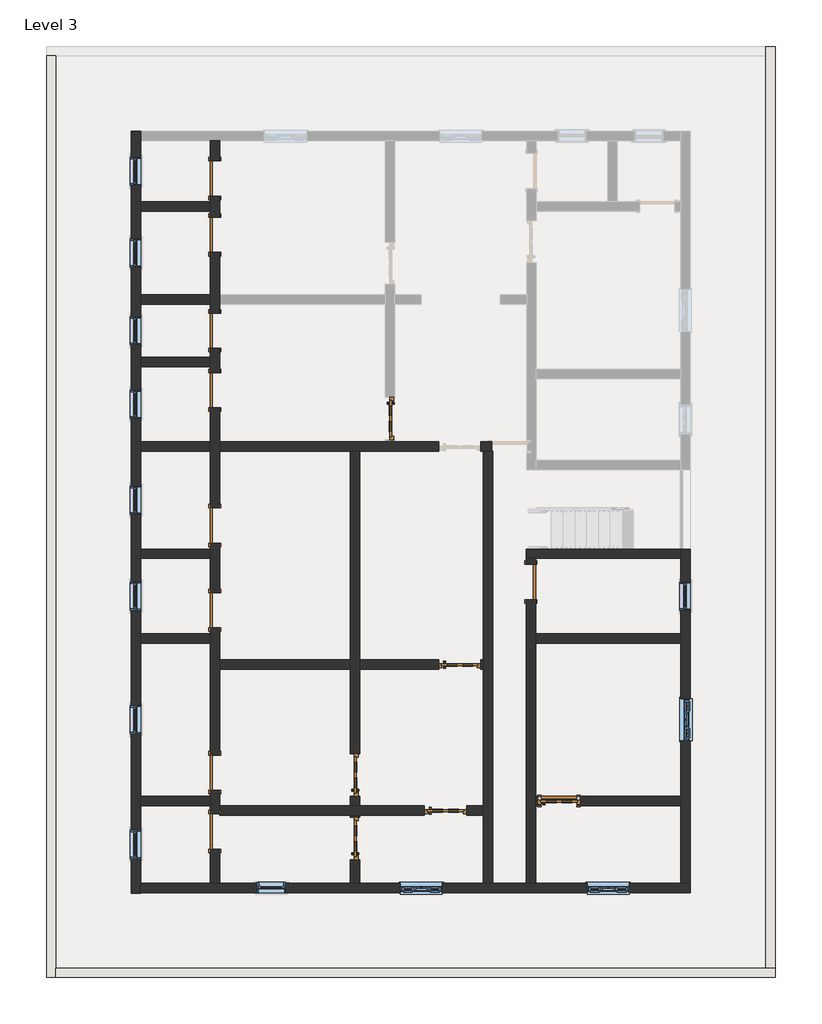
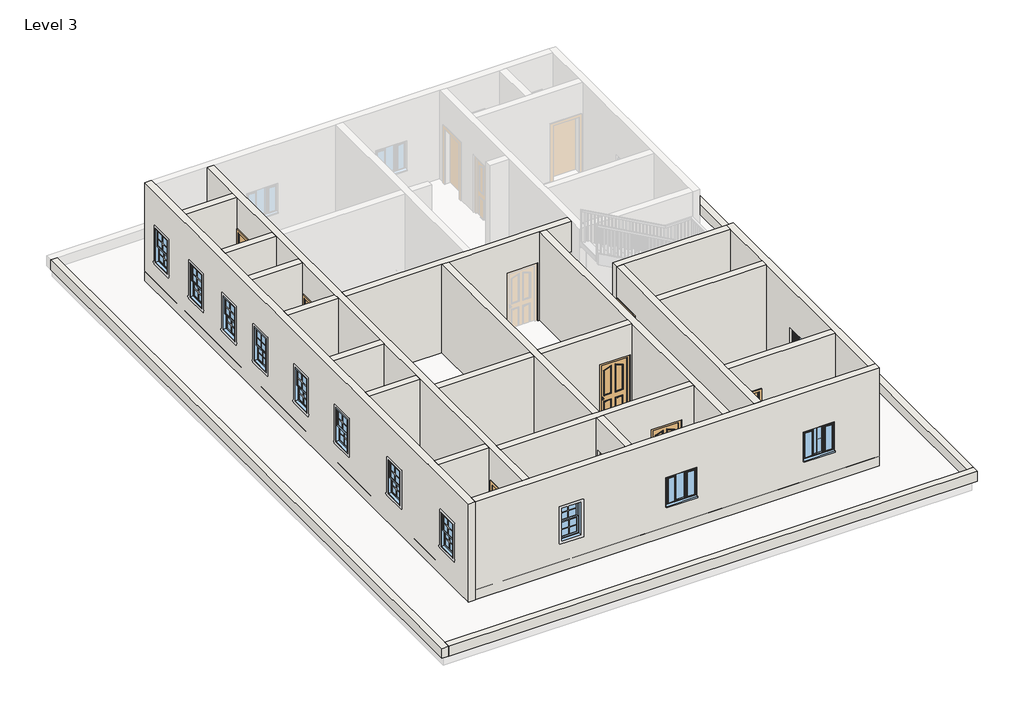
# One storey, part 1 of 3: 22 walls, 16 doors, 13 windows.
"""IFC4 building model written with IfcOpenShell, lengths in millimetres."""

from ifc_helpers import new_model, si_unit, frame, origin, place, context, project, spatial, polyline, outline, extrude, faceted_brep, transform, mapped, element, save
from components import doors_extsgl_12_910x2110mm_9a09825e, doors_extsgl_12_910x2110mm_ece77ece, door_fadea3f2, door_53b1b562, window_679d2811, windows_tpl_w_glazing_cross_bars_910x910mm_4aa0f884

model = new_model("IFC4")

# Units and contexts
model_context = context("Model", 3, world=origin())
ifc_project = project(units=[si_unit("LENGTHUNIT", "METRE", prefix="MILLI")], contexts=[model_context])

# Site, building, storey
site = spatial("IfcSite", under=ifc_project)
building = spatial("IfcBuilding", under=site)
storey = spatial("IfcBuildingStorey", under=building, Name="Level 3", Elevation=6096.0)

# Doors
placement = place(None, origin())
doors_extsgl_12_910x2110mm_shape = doors_extsgl_12_910x2110mm_9a09825e(model_context)
element("IfcDoor", 1, ObjectType="Doors_ExtSgl_12 : 910x2110mm", at=placement, inside=storey, context=model_context, shape_type="MappedRepresentation", body=[
    mapped(doors_extsgl_12_910x2110mm_shape, transform((-4887.6876145, 1213.3404944, 6096.0), x_axis=(0.0, -1.0, 0.0), y_axis=(1.0, 0.0, 0.0), z_axis=(0.0, 0.0, 1.0))),
])
doors_extsgl_12_910x2110mm_2_shape = doors_extsgl_12_910x2110mm_ece77ece(model_context)
element("IfcDoor", 2, ObjectType="Doors_ExtSgl_12 : 910x2110mm", at=placement, inside=storey, context=model_context, shape_type="MappedRepresentation", body=[
    mapped(doors_extsgl_12_910x2110mm_2_shape, transform((-5649.6876145, -6482.8595056, 6096.0), x_axis=(0.0, 1.0, 0.0), y_axis=(-1.0, 0.0, 0.0), z_axis=(0.0, 0.0, 1.0))),
])
element("IfcDoor", 3, ObjectType="Doors_ExtSgl_12 : 910x2110mm", at=placement, inside=storey, context=model_context, shape_type="MappedRepresentation", body=[
    mapped(doors_extsgl_12_910x2110mm_2_shape, transform((-1242.7876145, -7041.6595056, 6096.0), x_axis=(1.0, 0.0, 0.0), y_axis=(0.0, 1.0, 0.0), z_axis=(0.0, 0.0, 1.0))),
])
element("IfcDoor", 4, ObjectType="Doors_ExtSgl_12 : 910x2110mm", at=placement, inside=storey, context=model_context, shape_type="MappedRepresentation", body=[
    mapped(doors_extsgl_12_910x2110mm_2_shape, transform((-5649.6876145, -7854.4595056, 6096.0), x_axis=(0.0, 1.0, 0.0), y_axis=(-1.0, 0.0, 0.0), z_axis=(0.0, 0.0, 1.0))),
])
element("IfcDoor", 5, ObjectType="Doors_ExtSgl_12 : 910x2110mm", at=placement, inside=storey, context=model_context, shape_type="MappedRepresentation", body=[
    mapped(doors_extsgl_12_910x2110mm_2_shape, transform((-3693.8876145, -7244.8595056, 6096.0), x_axis=(1.0, 0.0, 0.0), y_axis=(0.0, 1.0, 0.0), z_axis=(0.0, 0.0, 1.0))),
])
element("IfcDoor", 6, ObjectType="Doors_ExtSgl_12 : 910x2110mm", at=placement, inside=storey, context=model_context, shape_type="MappedRepresentation", body=[
    mapped(doors_extsgl_12_910x2110mm_2_shape, transform((-3389.0876145, -4095.2595056, 6096.0), x_axis=(1.0, 0.0, 0.0), y_axis=(0.0, 1.0, 0.0), z_axis=(0.0, 0.0, 1.0))),
])
door_shape = door_fadea3f2(model_context)
element("IfcDoor", 7, ObjectType="Single-Flush : 30\" x 80\"", at=placement, inside=storey, context=model_context, shape_type="MappedRepresentation", body=[
    mapped(door_shape, transform((-8672.2876145, 5175.7404944, 6096.0), x_axis=(0.0, 1.0, 0.0), y_axis=(-1.0, 0.0, 0.0), z_axis=(0.0, 0.0, 1.0))),
])
element("IfcDoor", 8, ObjectType="Single-Flush : 30\" x 80\"", at=placement, inside=storey, context=model_context, shape_type="MappedRepresentation", body=[
    mapped(door_shape, transform((-8672.2876145, -7702.0595056, 6096.0), x_axis=(0.0, 1.0, 0.0), y_axis=(-1.0, 0.0, 0.0), z_axis=(0.0, 0.0, 1.0))),
])
element("IfcDoor", 9, ObjectType="Single-Flush : 30\" x 80\"", at=placement, inside=storey, context=model_context, shape_type="MappedRepresentation", body=[
    mapped(door_shape, transform((-1852.3876145, -2317.2595056, 6096.0), x_axis=(0.0, -1.0, 0.0), y_axis=(1.0, 0.0, 0.0), z_axis=(0.0, 0.0, 1.0))),
])
element("IfcDoor", 10, ObjectType="Single-Flush : 30\" x 80\"", at=placement, inside=storey, context=model_context, shape_type="MappedRepresentation", body=[
    mapped(door_shape, transform((-1242.7876145, -7041.6595056, 6096.0), x_axis=(1.0, 0.0, 0.0), y_axis=(0.0, 1.0, 0.0), z_axis=(0.0, 0.0, 1.0))),
])
door_2_shape = door_53b1b562(model_context)
element("IfcDoor", 11, ObjectType="Single-Flush : 30\" x 80\"", at=placement, inside=storey, context=model_context, shape_type="MappedRepresentation", body=[
    mapped(door_2_shape, transform((-8672.2876145, 6394.9404944, 6096.0), x_axis=(0.0, -1.0, 0.0), y_axis=(1.0, 0.0, 0.0), z_axis=(0.0, 0.0, 1.0))),
])
element("IfcDoor", 12, ObjectType="Single-Flush : 30\" x 80\"", at=placement, inside=storey, context=model_context, shape_type="MappedRepresentation", body=[
    mapped(door_2_shape, transform((-8672.2876145, 3105.6404944, 6096.0), x_axis=(0.0, -1.0, 0.0), y_axis=(1.0, 0.0, 0.0), z_axis=(0.0, 0.0, 1.0))),
])
element("IfcDoor", 13, ObjectType="Single-Flush : 30\" x 80\"", at=placement, inside=storey, context=model_context, shape_type="MappedRepresentation", body=[
    mapped(door_2_shape, transform((-8672.2876145, 1822.9404944, 6096.0), x_axis=(0.0, -1.0, 0.0), y_axis=(1.0, 0.0, 0.0), z_axis=(0.0, 0.0, 1.0))),
])
element("IfcDoor", 14, ObjectType="Single-Flush : 30\" x 80\"", at=placement, inside=storey, context=model_context, shape_type="MappedRepresentation", body=[
    mapped(door_2_shape, transform((-8672.2876145, -1098.0595056, 6096.0), x_axis=(0.0, -1.0, 0.0), y_axis=(1.0, 0.0, 0.0), z_axis=(0.0, 0.0, 1.0))),
])
element("IfcDoor", 15, ObjectType="Single-Flush : 30\" x 80\"", at=placement, inside=storey, context=model_context, shape_type="MappedRepresentation", body=[
    mapped(door_2_shape, transform((-8672.2876145, -2926.8595056, 6096.0), x_axis=(0.0, -1.0, 0.0), y_axis=(1.0, 0.0, 0.0), z_axis=(0.0, 0.0, 1.0))),
])
element("IfcDoor", 16, ObjectType="Single-Flush : 30\" x 80\"", at=placement, inside=storey, context=model_context, shape_type="MappedRepresentation", body=[
    mapped(door_2_shape, transform((-8672.2876145, -6432.0595056, 6096.0), x_axis=(0.0, -1.0, 0.0), y_axis=(1.0, 0.0, 0.0), z_axis=(0.0, 0.0, 1.0))),
])

# Walls
element("IfcWall", 17, ObjectType="4.5\"", at=placement, inside=storey, context=model_context, shape_type="Brep", body=[
    faceted_brep([(-8773.8876145, -6813.0595056, 6096.0), (-8773.8876145, -6940.0595056, 6096.0), (-8773.8876145, -7143.2595056, 6096.0), (-8773.8876145, -7321.0595056, 6096.0), (-8773.8876145, -7321.0595056, 8128.0), (-8773.8876145, -8083.0595056, 8128.0), (-8773.8876145, -8083.0595056, 6096.0), (-8773.8876145, -8819.6595056, 6096.0), (-8773.8876145, -8819.6595056, 9144.0), (-8773.8876145, -7143.2595056, 9144.0), (-8773.8876145, -6940.0595056, 9144.0), (-8773.8876145, -3638.0595056, 9144.0), (-8773.8876145, -3434.8595056, 9144.0), (-8773.8876145, -1809.2595056, 9144.0), (-8773.8876145, -1606.0595056, 9144.0), (-8773.8876145, 502.1404944, 9144.0), (-8773.8876145, 705.3404944, 9144.0), (-8773.8876145, 2330.9404944, 9144.0), (-8773.8876145, 2534.1404944, 9144.0), (-8773.8876145, 3677.1404944, 9144.0), (-8773.8876145, 3880.3404944, 9144.0), (-8773.8876145, 5683.7404944, 9144.0), (-8773.8876145, 5886.9404944, 9144.0), (-8773.8876145, 7207.7404944, 9144.0), (-8773.8876145, 7207.7404944, 6096.0), (-8773.8876145, 6775.9404944, 6096.0), (-8773.8876145, 6775.9404944, 8128.0), (-8773.8876145, 6013.9404944, 8128.0), (-8773.8876145, 6013.9404944, 6096.0), (-8773.8876145, 5886.9404944, 6096.0), (-8773.8876145, 5683.7404944, 6096.0), (-8773.8876145, 5556.7404944, 6096.0), (-8773.8876145, 5556.7404944, 8128.0), (-8773.8876145, 4794.7404944, 8128.0), (-8773.8876145, 4794.7404944, 6096.0), (-8773.8876145, 3880.3404944, 6096.0), (-8773.8876145, 3677.1404944, 6096.0), (-8773.8876145, 3486.6404944, 6096.0), (-8773.8876145, 3486.6404944, 8128.0), (-8773.8876145, 2724.6404944, 8128.0), (-8773.8876145, 2724.6404944, 6096.0), (-8773.8876145, 2534.1404944, 6096.0), (-8773.8876145, 2330.9404944, 6096.0), (-8773.8876145, 2203.9404944, 6096.0), (-8773.8876145, 2203.9404944, 8128.0), (-8773.8876145, 1441.9404944, 8128.0), (-8773.8876145, 1441.9404944, 6096.0), (-8773.8876145, 705.3404944, 6096.0), (-8773.8876145, 502.1404944, 6096.0), (-8773.8876145, -717.0595056, 6096.0), (-8773.8876145, -717.0595056, 8128.0), (-8773.8876145, -1479.0595056, 8128.0), (-8773.8876145, -1479.0595056, 6096.0), (-8773.8876145, -1606.0595056, 6096.0), (-8773.8876145, -1809.2595056, 6096.0), (-8773.8876145, -2545.8595056, 6096.0), (-8773.8876145, -2545.8595056, 8128.0), (-8773.8876145, -3307.8595056, 8128.0), (-8773.8876145, -3307.8595056, 6096.0), (-8773.8876145, -3434.8595056, 6096.0), (-8773.8876145, -3638.0595056, 6096.0), (-8773.8876145, -6051.0595056, 6096.0), (-8773.8876145, -6051.0595056, 8128.0), (-8773.8876145, -6813.0595056, 8128.0), (-8570.6876145, -7321.0595056, 8128.0), (-8570.6876145, -7321.0595056, 6096.0), (-8570.6876145, -7143.2595056, 6096.0), (-8570.6876145, -6813.0595056, 6096.0), (-8570.6876145, -6813.0595056, 8128.0), (-8570.6876145, -6051.0595056, 8128.0), (-8570.6876145, -6051.0595056, 6096.0), (-8570.6876145, -4196.8595056, 6096.0), (-8570.6876145, -3993.6595056, 6096.0), (-8570.6876145, -3307.8595056, 6096.0), (-8570.6876145, -3307.8595056, 8128.0), (-8570.6876145, -2545.8595056, 8128.0), (-8570.6876145, -2545.8595056, 6096.0), (-8570.6876145, -1479.0595056, 6096.0), (-8570.6876145, -1479.0595056, 8128.0), (-8570.6876145, -717.0595056, 8128.0), (-8570.6876145, -717.0595056, 6096.0), (-8570.6876145, 502.1404944, 6096.0), (-8570.6876145, 705.3404944, 6096.0), (-8570.6876145, 1441.9404944, 6096.0), (-8570.6876145, 1441.9404944, 8128.0), (-8570.6876145, 2203.9404944, 8128.0), (-8570.6876145, 2203.9404944, 6096.0), (-8570.6876145, 2724.6404944, 6096.0), (-8570.6876145, 2724.6404944, 8128.0), (-8570.6876145, 3486.6404944, 8128.0), (-8570.6876145, 3486.6404944, 6096.0), (-8570.6876145, 3677.1404944, 6096.0), (-8570.6876145, 3880.3404944, 6096.0), (-8570.6876145, 4794.7404944, 6096.0), (-8570.6876145, 4794.7404944, 8128.0), (-8570.6876145, 5556.7404944, 8128.0), (-8570.6876145, 5556.7404944, 6096.0), (-8570.6876145, 6013.9404944, 6096.0), (-8570.6876145, 6013.9404944, 8128.0), (-8570.6876145, 6775.9404944, 8128.0), (-8570.6876145, 6775.9404944, 6096.0), (-8570.6876145, 7207.7404944, 6096.0), (-8570.6876145, 7207.7404944, 9144.0), (-8570.6876145, 3880.3404944, 9144.0), (-8570.6876145, 3677.1404944, 9144.0), (-8570.6876145, 705.3404944, 9144.0), (-8570.6876145, 502.1404944, 9144.0), (-8570.6876145, -3993.6595056, 9144.0), (-8570.6876145, -4196.8595056, 9144.0), (-8570.6876145, -7143.2595056, 9144.0), (-8570.6876145, -7346.4595056, 9144.0), (-8570.6876145, -8819.6595056, 9144.0), (-8570.6876145, -8819.6595056, 6096.0), (-8570.6876145, -8083.0595056, 6096.0), (-8570.6876145, -8083.0595056, 8128.0)], [[[0, 1, 2, 3, 4, 5, 6, 7, 8, 9, 10, 11, 12, 13, 14, 15, 16, 17, 18, 19, 20, 21, 22, 23, 24, 25, 26, 27, 28, 29, 30, 31, 32, 33, 34, 35, 36, 37, 38, 39, 40, 41, 42, 43, 44, 45, 46, 47, 48, 49, 50, 51, 52, 53, 54, 55, 56, 57, 58, 59, 60, 61, 62, 63]], [[64, 65, 66, 67, 68, 69, 70, 71, 72, 73, 74, 75, 76, 77, 78, 79, 80, 81, 82, 83, 84, 85, 86, 87, 88, 89, 90, 91, 92, 93, 94, 95, 96, 97, 98, 99, 100, 101, 102, 103, 104, 105, 106, 107, 108, 109, 110, 111, 112, 113, 114]], [[25, 24, 101, 100]], [[97, 96, 31, 30, 29, 28]], [[37, 36, 35, 34, 93, 92, 91, 90]], [[43, 42, 41, 40, 87, 86]], [[49, 48, 47, 46, 83, 82, 81, 80]], [[55, 54, 53, 52, 77, 76]], [[61, 60, 59, 58, 73, 72, 71, 70]], [[113, 112, 7, 6]], [[67, 66, 65, 3, 2, 1, 0]], [[23, 22, 21, 20, 19, 18, 17, 16, 15, 14, 13, 12, 11, 10, 9, 8, 111, 110, 109, 108, 107, 106, 105, 104, 103, 102]], [[8, 7, 112, 111]], [[24, 23, 102, 101]], [[98, 97, 28, 27]], [[99, 98, 27, 26]], [[100, 99, 26, 25]], [[32, 31, 96, 95]], [[33, 32, 95, 94]], [[34, 33, 94, 93]], [[88, 87, 40, 39]], [[89, 88, 39, 38]], [[90, 89, 38, 37]], [[84, 83, 46, 45]], [[85, 84, 45, 44]], [[86, 85, 44, 43]], [[78, 77, 52, 51]], [[79, 78, 51, 50]], [[80, 79, 50, 49]], [[74, 73, 58, 57]], [[75, 74, 57, 56]], [[76, 75, 56, 55]], [[68, 67, 0, 63]], [[69, 68, 63, 62]], [[70, 69, 62, 61]], [[4, 3, 65, 64]], [[5, 4, 64, 114]], [[6, 5, 114, 113]]]),
])
element("IfcWall", 18, ObjectType="4.5\"", at=placement, inside=storey, context=model_context, shape_type="SweptSolid", body=[
    extrude(outline(polyline([(-8773.8876145, 5683.7404944), (-10272.4876145, 5683.7404944), (-10272.4876145, 5886.9404944), (-8773.8876145, 5886.9404944), (-8773.8876145, 5683.7404944)])), frame((0.0, 0.0, 6096.0), z_axis=(0.0, 0.0, 1.0), x_axis=(1.0, 0.0, 0.0)), (0.0, 0.0, 1.0), 3048.0),
])
element("IfcWall", 19, ObjectType="4.5\"", at=placement, inside=storey, context=model_context, shape_type="SweptSolid", body=[
    extrude(outline(polyline([(-8773.8876145, 3677.1404944), (-10272.4876145, 3677.1404944), (-10272.4876145, 3880.3404944), (-8773.8876145, 3880.3404944), (-8773.8876145, 3677.1404944)])), frame((0.0, 0.0, 6096.0), z_axis=(0.0, 0.0, 1.0), x_axis=(1.0, 0.0, 0.0)), (0.0, 0.0, 1.0), 3048.0),
])
element("IfcWall", 20, ObjectType="4.5\"", at=placement, inside=storey, context=model_context, shape_type="SweptSolid", body=[
    extrude(outline(polyline([(-8773.8876145, 2330.9404944), (-10272.4876145, 2330.9404944), (-10272.4876145, 2534.1404944), (-8773.8876145, 2534.1404944), (-8773.8876145, 2330.9404944)])), frame((0.0, 0.0, 6096.0), z_axis=(0.0, 0.0, 1.0), x_axis=(1.0, 0.0, 0.0)), (0.0, 0.0, 1.0), 3048.0),
])
element("IfcWall", 21, ObjectType="4.5\"", at=placement, inside=storey, context=model_context, shape_type="Brep", body=[
    faceted_brep([(-10272.4876145, 502.1404944, 9144.0), (-10272.4876145, 502.1404944, 6096.0), (-8773.8876145, 502.1404944, 6096.0), (-8773.8876145, 502.1404944, 9144.0), (-10272.4876145, 705.3404944, 6096.0), (-10272.4876145, 705.3404944, 9144.0), (-8773.8876145, 705.3404944, 9144.0), (-8773.8876145, 705.3404944, 6096.0)], [[[0, 1, 2, 3]], [[4, 5, 6, 7]], [[1, 4, 7, 2]], [[5, 0, 3, 6]], [[1, 0, 5, 4]], [[3, 2, 7, 6]]]),
    faceted_brep([(-1941.2876145, 502.1404944, 8128.0), (-1941.2876145, 502.1404944, 9144.0), (-2677.8876145, 502.1404944, 9144.0), (-2881.0876145, 502.1404944, 9144.0), (-5548.0876145, 502.1404944, 9144.0), (-5751.2876145, 502.1404944, 9144.0), (-8570.6876145, 502.1404944, 9144.0), (-8570.6876145, 502.1404944, 6096.0), (-5751.2876145, 502.1404944, 6096.0), (-5548.0876145, 502.1404944, 6096.0), (-3844.0876145, 502.1404944, 6096.0), (-3844.0876145, 502.1404944, 8206.0), (-2934.0876145, 502.1404944, 8206.0), (-2934.0876145, 502.1404944, 6096.0), (-2881.0876145, 502.1404944, 6096.0), (-2690.5876145, 502.1404944, 6096.0), (-2690.5876145, 502.1404944, 8128.0), (-1941.2876145, 705.3404944, 9144.0), (-1941.2876145, 705.3404944, 8128.0), (-2690.5876145, 705.3404944, 8128.0), (-2690.5876145, 705.3404944, 6096.0), (-2934.0876145, 705.3404944, 6096.0), (-2934.0876145, 705.3404944, 8206.0), (-3844.0876145, 705.3404944, 8206.0), (-3844.0876145, 705.3404944, 6096.0), (-4786.0876145, 705.3404944, 6096.0), (-4989.2876145, 705.3404944, 6096.0), (-8570.6876145, 705.3404944, 6096.0), (-8570.6876145, 705.3404944, 9144.0), (-4989.2876145, 705.3404944, 9144.0), (-4786.0876145, 705.3404944, 9144.0)], [[[0, 1, 2, 3, 4, 5, 6, 7, 8, 9, 10, 11, 12, 13, 14, 15, 16]], [[17, 18, 19, 20, 21, 22, 23, 24, 25, 26, 27, 28, 29, 30]], [[20, 15, 14, 13, 21]], [[24, 10, 9, 8, 7, 27, 26, 25]], [[1, 17, 30, 29, 28, 6, 5, 4, 3, 2]], [[7, 6, 28, 27]], [[17, 1, 0, 18]], [[16, 19, 18, 0]], [[19, 16, 15, 20]], [[24, 23, 11, 10]], [[22, 21, 13, 12]], [[23, 22, 12, 11]]]),
])
element("IfcWall", 22, ObjectType="4.5\"", at=placement, inside=storey, context=model_context, shape_type="SweptSolid", body=[
    extrude(outline(polyline([(-8773.8876145, -1809.2595056), (-10272.4876145, -1809.2595056), (-10272.4876145, -1606.0595056), (-8773.8876145, -1606.0595056), (-8773.8876145, -1809.2595056)])), frame((0.0, 0.0, 6096.0), z_axis=(0.0, 0.0, 1.0), x_axis=(1.0, 0.0, 0.0)), (0.0, 0.0, 1.0), 3048.0),
])
element("IfcWall", 23, ObjectType="4.5\"", at=placement, inside=storey, context=model_context, shape_type="SweptSolid", body=[
    extrude(outline(polyline([(-8773.8876145, -3638.0595056), (-10272.4876145, -3638.0595056), (-10272.4876145, -3434.8595056), (-8773.8876145, -3434.8595056), (-8773.8876145, -3638.0595056)])), frame((0.0, 0.0, 6096.0), z_axis=(0.0, 0.0, 1.0), x_axis=(1.0, 0.0, 0.0)), (0.0, 0.0, 1.0), 3048.0),
])
element("IfcWall", 24, ObjectType="4.5\"", at=placement, inside=storey, context=model_context, shape_type="SweptSolid", body=[
    extrude(outline(polyline([(-8773.8876145, -7143.2595056), (-10272.4876145, -7143.2595056), (-10272.4876145, -6940.0595056), (-8773.8876145, -6940.0595056), (-8773.8876145, -7143.2595056)])), frame((0.0, 0.0, 6096.0), z_axis=(0.0, 0.0, 1.0), x_axis=(1.0, 0.0, 0.0)), (0.0, 0.0, 1.0), 3048.0),
])
element("IfcWall", 25, ObjectType="4.5\"", at=placement, inside=storey, context=model_context, shape_type="Brep", body=[
    faceted_brep([(-3238.8876145, -7346.4595056, 8206.0), (-3238.8876145, -7346.4595056, 6096.0), (-2881.0876145, -7346.4595056, 6096.0), (-2881.0876145, -7346.4595056, 9144.0), (-5548.0876145, -7346.4595056, 9144.0), (-5751.2876145, -7346.4595056, 9144.0), (-8570.6876145, -7346.4595056, 9144.0), (-8570.6876145, -7346.4595056, 6096.0), (-5751.2876145, -7346.4595056, 6096.0), (-5548.0876145, -7346.4595056, 6096.0), (-4148.8876145, -7346.4595056, 6096.0), (-4148.8876145, -7346.4595056, 8206.0), (-2881.0876145, -7143.2595056, 6096.0), (-3238.8876145, -7143.2595056, 6096.0), (-3238.8876145, -7143.2595056, 8206.0), (-4148.8876145, -7143.2595056, 8206.0), (-4148.8876145, -7143.2595056, 6096.0), (-5548.0876145, -7143.2595056, 6096.0), (-5751.2876145, -7143.2595056, 6096.0), (-8570.6876145, -7143.2595056, 6096.0), (-8570.6876145, -7143.2595056, 9144.0), (-5751.2876145, -7143.2595056, 9144.0), (-5548.0876145, -7143.2595056, 9144.0), (-2881.0876145, -7143.2595056, 9144.0), (-8570.6876145, -7321.0595056, 6096.0)], [[[0, 1, 2, 3, 4, 5, 6, 7, 8, 9, 10, 11]], [[12, 13, 14, 15, 16, 17, 18, 19, 20, 21, 22, 23]], [[2, 1, 13, 12]], [[10, 9, 8, 7, 24, 19, 18, 17, 16]], [[6, 5, 4, 3, 23, 22, 21, 20]], [[7, 6, 20, 19, 24]], [[3, 2, 12, 23]], [[16, 15, 11, 10]], [[14, 13, 1, 0]], [[15, 14, 0, 11]]]),
])
element("IfcWall", 26, ObjectType="4.5\"", at=placement, inside=storey, context=model_context, shape_type="Brep", body=[
    faceted_brep([(-5751.2876145, -8819.6595056, 6096.0), (-5751.2876145, -8819.6595056, 9144.0), (-5751.2876145, -7346.4595056, 9144.0), (-5751.2876145, -7346.4595056, 6096.0), (-5751.2876145, -7399.4595056, 6096.0), (-5751.2876145, -7399.4595056, 8206.0), (-5751.2876145, -8309.4595056, 8206.0), (-5751.2876145, -8309.4595056, 6096.0), (-5548.0876145, -8819.6595056, 9144.0), (-5548.0876145, -8819.6595056, 6096.0), (-5548.0876145, -8309.4595056, 6096.0), (-5548.0876145, -8309.4595056, 8206.0), (-5548.0876145, -7399.4595056, 8206.0), (-5548.0876145, -7399.4595056, 6096.0), (-5548.0876145, -7346.4595056, 6096.0), (-5548.0876145, -7346.4595056, 9144.0)], [[[0, 1, 2, 3, 4, 5, 6, 7]], [[8, 9, 10, 11, 12, 13, 14, 15]], [[9, 0, 7, 10]], [[13, 4, 3, 14]], [[1, 8, 15, 2]], [[1, 0, 9, 8]], [[3, 2, 15, 14]], [[7, 6, 11, 10]], [[5, 4, 13, 12]], [[6, 5, 12, 11]]]),
    faceted_brep([(-5751.2876145, 502.1404944, 9144.0), (-5751.2876145, 502.1404944, 6096.0), (-5751.2876145, -3993.6595056, 6096.0), (-5751.2876145, -4196.8595056, 6096.0), (-5751.2876145, -6027.8595056, 6096.0), (-5751.2876145, -6027.8595056, 8206.0), (-5751.2876145, -6937.8595056, 8206.0), (-5751.2876145, -6937.8595056, 6096.0), (-5751.2876145, -7143.2595056, 6096.0), (-5751.2876145, -7143.2595056, 9144.0), (-5751.2876145, -4196.8595056, 9144.0), (-5751.2876145, -3993.6595056, 9144.0), (-5548.0876145, 502.1404944, 6096.0), (-5548.0876145, 502.1404944, 9144.0), (-5548.0876145, -3993.6595056, 9144.0), (-5548.0876145, -4196.8595056, 9144.0), (-5548.0876145, -7143.2595056, 9144.0), (-5548.0876145, -7143.2595056, 6096.0), (-5548.0876145, -6937.8595056, 6096.0), (-5548.0876145, -6937.8595056, 8206.0), (-5548.0876145, -6027.8595056, 8206.0), (-5548.0876145, -6027.8595056, 6096.0), (-5548.0876145, -4196.8595056, 6096.0), (-5548.0876145, -3993.6595056, 6096.0)], [[[0, 1, 2, 3, 4, 5, 6, 7, 8, 9, 10, 11]], [[12, 13, 14, 15, 16, 17, 18, 19, 20, 21, 22, 23]], [[1, 12, 23, 22, 21, 4, 3, 2]], [[7, 18, 17, 8]], [[13, 0, 11, 10, 9, 16, 15, 14]], [[1, 0, 13, 12]], [[9, 8, 17, 16]], [[7, 6, 19, 18]], [[5, 4, 21, 20]], [[6, 5, 20, 19]]]),
])
element("IfcWall", 27, ObjectType="4.5\"", at=placement, inside=storey, context=model_context, shape_type="SweptSolid", body=[
    extrude(outline(polyline([(-8570.6876145, -4196.8595056), (-8570.6876145, -3993.6595056), (-5751.2876145, -3993.6595056), (-5751.2876145, -4196.8595056), (-8570.6876145, -4196.8595056)])), frame((0.0, 0.0, 6096.0), z_axis=(0.0, 0.0, 1.0), x_axis=(1.0, 0.0, 0.0)), (0.0, 0.0, 1.0), 3048.0),
    extrude(outline(polyline([(6096.0, -2881.0876145), (9144.0, -2881.0876145), (9144.0, -5548.0876145), (6096.0, -5548.0876145), (6096.0, -3844.0876145), (8206.0, -3844.0876145), (8206.0, -2934.0876145), (6096.0, -2934.0876145), (6096.0, -2881.0876145)])), frame((0.0, -4196.8595056, 0.0), z_axis=(0.0, 1.0, 0.0), x_axis=(0.0, 0.0, 1.0)), (0.0, 0.0, 1.0), 203.2),
])
element("IfcWall", 28, ObjectType="4.5\"", at=placement, inside=storey, context=model_context, shape_type="Brep", body=[
    faceted_brep([(-2881.0876145, 502.1404944, 6096.0), (-2881.0876145, -3993.6595056, 6096.0), (-2881.0876145, -4196.8595056, 6096.0), (-2881.0876145, -7143.2595056, 6096.0), (-2881.0876145, -7346.4595056, 6096.0), (-2881.0876145, -8819.6595056, 6096.0), (-2881.0876145, -8819.6595056, 9144.0), (-2881.0876145, -7346.4595056, 9144.0), (-2881.0876145, -7143.2595056, 9144.0), (-2881.0876145, -4196.8595056, 9144.0), (-2881.0876145, -3993.6595056, 9144.0), (-2881.0876145, 502.1404944, 9144.0), (-2677.8876145, 502.1404944, 6096.0), (-2677.8876145, 502.1404944, 9144.0), (-2677.8876145, -8819.6595056, 9144.0), (-2677.8876145, -8819.6595056, 6096.0), (-2690.5876145, 502.1404944, 6096.0)], [[[0, 1, 2, 3, 4, 5, 6, 7, 8, 9, 10, 11]], [[12, 13, 14, 15]], [[5, 4, 3, 2, 1, 0, 16, 12, 15]], [[11, 10, 9, 8, 7, 6, 14, 13]], [[6, 5, 15, 14]], [[0, 11, 13, 12, 16]]]),
])
element("IfcWall", 29, ObjectType="4.5\"", at=placement, inside=storey, context=model_context, shape_type="Brep", body=[
    faceted_brep([(1386.1123855, -1606.0595056, 6096.0), (-1953.9876145, -1606.0595056, 6096.0), (-1953.9876145, -1606.0595056, 9144.0), (1386.1123855, -1606.0595056, 9144.0), (1386.1123855, -1809.2595056, 6096.0), (1386.1123855, -1809.2595056, 9144.0), (-1750.7876145, -1809.2595056, 9144.0), (-1953.9876145, -1809.2595056, 9144.0), (-1953.9876145, -1809.2595056, 6096.0), (-1750.7876145, -1809.2595056, 6096.0)], [[[0, 1, 2, 3]], [[4, 5, 6, 7, 8, 9]], [[1, 0, 4, 9, 8]], [[3, 2, 7, 6, 5]], [[0, 3, 5, 4]], [[2, 1, 8, 7]]]),
])
element("IfcWall", 30, ObjectType="4.5\"", at=placement, inside=storey, context=model_context, shape_type="Brep", body=[
    faceted_brep([(-1953.9876145, -2698.2595056, 8128.0), (-1953.9876145, -2698.2595056, 6096.0), (-1953.9876145, -8819.6595056, 6096.0), (-1953.9876145, -8819.6595056, 9144.0), (-1953.9876145, -1809.2595056, 9144.0), (-1953.9876145, -1809.2595056, 6096.0), (-1953.9876145, -1936.2595056, 6096.0), (-1953.9876145, -1936.2595056, 8128.0), (-1750.7876145, -8819.6595056, 6096.0), (-1750.7876145, -7143.2595056, 6096.0), (-1750.7876145, -6940.0595056, 6096.0), (-1750.7876145, -3638.0595056, 6096.0), (-1750.7876145, -3434.8595056, 6096.0), (-1750.7876145, -2698.2595056, 6096.0), (-1750.7876145, -2698.2595056, 8128.0), (-1750.7876145, -1936.2595056, 8128.0), (-1750.7876145, -1936.2595056, 6096.0), (-1750.7876145, -1809.2595056, 6096.0), (-1750.7876145, -1809.2595056, 9144.0), (-1750.7876145, -3434.8595056, 9144.0), (-1750.7876145, -3638.0595056, 9144.0), (-1750.7876145, -6940.0595056, 9144.0), (-1750.7876145, -7143.2595056, 9144.0), (-1750.7876145, -8819.6595056, 9144.0)], [[[0, 1, 2, 3, 4, 5, 6, 7]], [[8, 9, 10, 11, 12, 13, 14, 15, 16, 17, 18, 19, 20, 21, 22, 23]], [[6, 5, 17, 16]], [[2, 1, 13, 12, 11, 10, 9, 8]], [[4, 3, 23, 22, 21, 20, 19, 18]], [[5, 4, 18, 17]], [[3, 2, 8, 23]], [[14, 13, 1, 0]], [[15, 14, 0, 7]], [[16, 15, 7, 6]]]),
])
element("IfcWall", 31, ObjectType="4.5\"", at=placement, inside=storey, context=model_context, shape_type="SweptSolid", body=[
    extrude(outline(polyline([(9144.0, 1386.1123855), (9144.0, -1750.7876145), (6096.0, -1750.7876145), (6096.0, -1697.7876145), (8206.0, -1697.7876145), (8206.0, -787.7876145), (6096.0, -787.7876145), (6096.0, 1386.1123855), (9144.0, 1386.1123855)])), frame((0.0, -7143.2595056, 0.0), z_axis=(0.0, 1.0, 0.0), x_axis=(0.0, 0.0, 1.0)), (0.0, 0.0, 1.0), 203.2),
])
element("IfcWall", 32, ObjectType="4.5\"", at=placement, inside=storey, context=model_context, shape_type="SweptSolid", body=[
    extrude(outline(polyline([(1386.1123855, -3638.0595056), (-1750.7876145, -3638.0595056), (-1750.7876145, -3434.8595056), (1386.1123855, -3434.8595056), (1386.1123855, -3638.0595056)])), frame((0.0, 0.0, 6096.0), z_axis=(0.0, 0.0, 1.0), x_axis=(1.0, 0.0, 0.0)), (0.0, 0.0, 1.0), 3048.0),
])
element("IfcWall", 33, ObjectType="4.5\"", at=placement, inside=storey, context=model_context, shape_type="Brep", body=[
    faceted_brep([(-12101.2876145, -10851.6595056, 6096.0), (-12101.2876145, -10648.4595056, 6096.0), (-12101.2876145, 9036.5404944, 6096.0), (-12101.2876145, 9036.5404944, 6400.8), (-12101.2876145, -10648.4595056, 6400.8), (-12101.2876145, -10851.6595056, 6400.8), (-12304.4876145, -10851.6595056, 6096.0), (-12304.4876145, -10851.6595056, 6400.8), (-12304.4876145, 9036.5404944, 6400.8), (-12304.4876145, 9036.5404944, 6096.0)], [[[0, 1, 2, 3, 4, 5]], [[6, 7, 8, 9]], [[2, 1, 0, 6, 9]], [[5, 4, 3, 8, 7]], [[0, 5, 7, 6]], [[3, 2, 9, 8]]]),
])
element("IfcWall", 34, ObjectType="4.5\"", at=placement, inside=storey, context=model_context, shape_type="Brep", body=[
    faceted_brep([(3418.1123855, -10648.4595056, 6096.0), (3214.9123855, -10648.4595056, 6096.0), (-12101.2876145, -10648.4595056, 6096.0), (-12101.2876145, -10648.4595056, 6400.8), (3214.9123855, -10648.4595056, 6400.8), (3418.1123855, -10648.4595056, 6400.8), (3418.1123855, -10851.6595056, 6096.0), (3418.1123855, -10851.6595056, 6400.8), (-12101.2876145, -10851.6595056, 6400.8), (-12101.2876145, -10851.6595056, 6096.0)], [[[0, 1, 2, 3, 4, 5]], [[6, 7, 8, 9]], [[2, 1, 0, 6, 9]], [[5, 4, 3, 8, 7]], [[0, 5, 7, 6]], [[3, 2, 9, 8]]]),
])
element("IfcWall", 35, ObjectType="4.5\"", at=placement, inside=storey, context=model_context, shape_type="Brep", body=[
    faceted_brep([(3214.9123855, 9239.7404944, 6096.0), (3214.9123855, 9036.5404944, 6096.0), (3214.9123855, -10648.4595056, 6096.0), (3214.9123855, -10648.4595056, 6400.8), (3214.9123855, 9036.5404944, 6400.8), (3214.9123855, 9239.7404944, 6400.8), (3418.1123855, 9239.7404944, 6096.0), (3418.1123855, 9239.7404944, 6400.8), (3418.1123855, -10648.4595056, 6400.8), (3418.1123855, -10648.4595056, 6096.0)], [[[0, 1, 2, 3, 4, 5]], [[6, 7, 8, 9]], [[2, 1, 0, 6, 9]], [[5, 4, 3, 8, 7]], [[0, 5, 7, 6]], [[3, 2, 9, 8]]]),
])
element("IfcWall", 36, ObjectType="Generic - 9\"", at=placement, inside=storey, context=model_context, shape_type="Brep", body=[
    faceted_brep([(-10475.6876145, 7410.9404944, 6096.0), (-10475.6876145, -9035.5595056, 6096.0), (-10475.6876145, -9035.5595056, 9144.0), (-10475.6876145, 7410.9404944, 9144.0), (-10475.6876145, 6242.5404944, 8077.2), (-10475.6876145, 6242.5404944, 7010.4), (-10475.6876145, 6852.1404944, 7010.4), (-10475.6876145, 6852.1404944, 8077.2), (-10475.6876145, 4477.2404944, 8077.2), (-10475.6876145, 4477.2404944, 7010.4), (-10475.6876145, 5086.8404944, 7010.4), (-10475.6876145, 5086.8404944, 8077.2), (-10475.6876145, 2800.8404944, 8077.2), (-10475.6876145, 2800.8404944, 7010.4), (-10475.6876145, 3410.4404944, 7010.4), (-10475.6876145, 3410.4404944, 8077.2), (-10475.6876145, 1213.3404944, 8077.2), (-10475.6876145, 1213.3404944, 7010.4), (-10475.6876145, 1822.9404944, 7010.4), (-10475.6876145, 1822.9404944, 8077.2), (-10475.6876145, -856.7595056, 8077.2), (-10475.6876145, -856.7595056, 7010.4), (-10475.6876145, -247.1595056, 7010.4), (-10475.6876145, -247.1595056, 8077.2), (-10475.6876145, -2926.8595056, 8077.2), (-10475.6876145, -2926.8595056, 7010.4), (-10475.6876145, -2317.2595056, 7010.4), (-10475.6876145, -2317.2595056, 8077.2), (-10475.6876145, -5593.8595056, 8077.2), (-10475.6876145, -5593.8595056, 7010.4), (-10475.6876145, -4984.2595056, 7010.4), (-10475.6876145, -4984.2595056, 8077.2), (-10475.6876145, -8286.2595056, 8077.2), (-10475.6876145, -8286.2595056, 7010.4), (-10475.6876145, -7676.6595056, 7010.4), (-10475.6876145, -7676.6595056, 8077.2), (-10272.4876145, 7410.9404944, 6096.0), (-10272.4876145, 7410.9404944, 9144.0), (-10272.4876145, 7207.7404944, 9144.0), (-10272.4876145, 5886.9404944, 9144.0), (-10272.4876145, 5683.7404944, 9144.0), (-10272.4876145, 3880.3404944, 9144.0), (-10272.4876145, 3677.1404944, 9144.0), (-10272.4876145, 2534.1404944, 9144.0), (-10272.4876145, 2330.9404944, 9144.0), (-10272.4876145, 705.3404944, 9144.0), (-10272.4876145, 502.1404944, 9144.0), (-10272.4876145, -1606.0595056, 9144.0), (-10272.4876145, -1809.2595056, 9144.0), (-10272.4876145, -3434.8595056, 9144.0), (-10272.4876145, -3638.0595056, 9144.0), (-10272.4876145, -6940.0595056, 9144.0), (-10272.4876145, -7143.2595056, 9144.0), (-10272.4876145, -8819.6595056, 9144.0), (-10272.4876145, -9022.8595056, 9144.0), (-10272.4876145, -9035.5595056, 9144.0), (-10272.4876145, -9035.5595056, 6096.0), (-10272.4876145, -9022.8595056, 6096.0), (-10272.4876145, -8819.6595056, 6096.0), (-10272.4876145, -7143.2595056, 6096.0), (-10272.4876145, -6940.0595056, 6096.0), (-10272.4876145, -3638.0595056, 6096.0), (-10272.4876145, -3434.8595056, 6096.0), (-10272.4876145, -1809.2595056, 6096.0), (-10272.4876145, -1606.0595056, 6096.0), (-10272.4876145, 502.1404944, 6096.0), (-10272.4876145, 705.3404944, 6096.0), (-10272.4876145, 2330.9404944, 6096.0), (-10272.4876145, 2534.1404944, 6096.0), (-10272.4876145, 3677.1404944, 6096.0), (-10272.4876145, 3880.3404944, 6096.0), (-10272.4876145, 5683.7404944, 6096.0), (-10272.4876145, 5886.9404944, 6096.0), (-10272.4876145, 7207.7404944, 6096.0), (-10272.4876145, 6242.5404944, 8077.2), (-10272.4876145, 6852.1404944, 8077.2), (-10272.4876145, 6852.1404944, 7010.4), (-10272.4876145, 6242.5404944, 7010.4), (-10272.4876145, 4477.2404944, 8077.2), (-10272.4876145, 5086.8404944, 8077.2), (-10272.4876145, 5086.8404944, 7010.4), (-10272.4876145, 4477.2404944, 7010.4), (-10272.4876145, 2800.8404944, 8077.2), (-10272.4876145, 3410.4404944, 8077.2), (-10272.4876145, 3410.4404944, 7010.4), (-10272.4876145, 2800.8404944, 7010.4), (-10272.4876145, 1213.3404944, 8077.2), (-10272.4876145, 1822.9404944, 8077.2), (-10272.4876145, 1822.9404944, 7010.4), (-10272.4876145, 1213.3404944, 7010.4), (-10272.4876145, -856.7595056, 8077.2), (-10272.4876145, -247.1595056, 8077.2), (-10272.4876145, -247.1595056, 7010.4), (-10272.4876145, -856.7595056, 7010.4), (-10272.4876145, -2926.8595056, 8077.2), (-10272.4876145, -2317.2595056, 8077.2), (-10272.4876145, -2317.2595056, 7010.4), (-10272.4876145, -2926.8595056, 7010.4), (-10272.4876145, -5593.8595056, 8077.2), (-10272.4876145, -4984.2595056, 8077.2), (-10272.4876145, -4984.2595056, 7010.4), (-10272.4876145, -5593.8595056, 7010.4), (-10272.4876145, -8286.2595056, 8077.2), (-10272.4876145, -7676.6595056, 8077.2), (-10272.4876145, -7676.6595056, 7010.4), (-10272.4876145, -8286.2595056, 7010.4)], [[[0, 1, 2, 3], [4, 5, 6, 7], [8, 9, 10, 11], [12, 13, 14, 15], [16, 17, 18, 19], [20, 21, 22, 23], [24, 25, 26, 27], [28, 29, 30, 31], [32, 33, 34, 35]], [[36, 37, 38, 39, 40, 41, 42, 43, 44, 45, 46, 47, 48, 49, 50, 51, 52, 53, 54, 55, 56, 57, 58, 59, 60, 61, 62, 63, 64, 65, 66, 67, 68, 69, 70, 71, 72, 73], [74, 75, 76, 77], [78, 79, 80, 81], [82, 83, 84, 85], [86, 87, 88, 89], [90, 91, 92, 93], [94, 95, 96, 97], [98, 99, 100, 101], [102, 103, 104, 105]], [[1, 0, 36, 73, 72, 71, 70, 69, 68, 67, 66, 65, 64, 63, 62, 61, 60, 59, 58, 57, 56]], [[2, 1, 56, 55]], [[3, 2, 55, 54, 53, 52, 51, 50, 49, 48, 47, 46, 45, 44, 43, 42, 41, 40, 39, 38, 37]], [[0, 3, 37, 36]], [[5, 4, 74, 77]], [[6, 5, 77, 76]], [[7, 6, 76, 75]], [[4, 7, 75, 74]], [[9, 8, 78, 81]], [[10, 9, 81, 80]], [[11, 10, 80, 79]], [[8, 11, 79, 78]], [[13, 12, 82, 85]], [[14, 13, 85, 84]], [[15, 14, 84, 83]], [[12, 15, 83, 82]], [[17, 16, 86, 89]], [[18, 17, 89, 88]], [[19, 18, 88, 87]], [[16, 19, 87, 86]], [[21, 20, 90, 93]], [[22, 21, 93, 92]], [[23, 22, 92, 91]], [[20, 23, 91, 90]], [[25, 24, 94, 97]], [[26, 25, 97, 96]], [[27, 26, 96, 95]], [[24, 27, 95, 94]], [[29, 28, 98, 101]], [[30, 29, 101, 100]], [[31, 30, 100, 99]], [[28, 31, 99, 98]], [[33, 32, 102, 105]], [[34, 33, 105, 104]], [[35, 34, 104, 103]], [[32, 35, 103, 102]]]),
])
element("IfcWall", 37, ObjectType="Generic - 9\"", at=placement, inside=storey, context=model_context, shape_type="Brep", body=[
    faceted_brep([(-10272.4876145, -9022.8595056, 6096.0), (1589.3123855, -9022.8595056, 6096.0), (1589.3123855, -9022.8595056, 9144.0), (-10272.4876145, -9022.8595056, 9144.0), (-7757.8876145, -9022.8595056, 8077.2), (-7148.2876145, -9022.8595056, 8077.2), (-7148.2876145, -9022.8595056, 7010.4), (-7757.8876145, -9022.8595056, 7010.4), (272.6623855, -9022.8595056, 7920.4), (272.6623855, -9022.8595056, 7010.4), (-637.3376145, -9022.8595056, 7010.4), (-637.3376145, -9022.8595056, 7920.4), (-3759.5876145, -9022.8595056, 7920.4), (-3759.5876145, -9022.8595056, 7010.4), (-4669.5876145, -9022.8595056, 7010.4), (-4669.5876145, -9022.8595056, 7920.4), (-10272.4876145, -8819.6595056, 6096.0), (-10272.4876145, -8819.6595056, 9144.0), (-8773.8876145, -8819.6595056, 9144.0), (-8570.6876145, -8819.6595056, 9144.0), (-5751.2876145, -8819.6595056, 9144.0), (-5548.0876145, -8819.6595056, 9144.0), (-2881.0876145, -8819.6595056, 9144.0), (-2677.8876145, -8819.6595056, 9144.0), (-1953.9876145, -8819.6595056, 9144.0), (-1750.7876145, -8819.6595056, 9144.0), (1386.1123855, -8819.6595056, 9144.0), (1589.3123855, -8819.6595056, 9144.0), (1589.3123855, -8819.6595056, 6096.0), (1386.1123855, -8819.6595056, 6096.0), (-1750.7876145, -8819.6595056, 6096.0), (-1953.9876145, -8819.6595056, 6096.0), (-2677.8876145, -8819.6595056, 6096.0), (-2881.0876145, -8819.6595056, 6096.0), (-5548.0876145, -8819.6595056, 6096.0), (-5751.2876145, -8819.6595056, 6096.0), (-8570.6876145, -8819.6595056, 6096.0), (-8773.8876145, -8819.6595056, 6096.0), (-7757.8876145, -8819.6595056, 8077.2), (-7757.8876145, -8819.6595056, 7010.4), (-7148.2876145, -8819.6595056, 7010.4), (-7148.2876145, -8819.6595056, 8077.2), (272.6623855, -8819.6595056, 7920.4), (-637.3376145, -8819.6595056, 7920.4), (-637.3376145, -8819.6595056, 7010.4), (272.6623855, -8819.6595056, 7010.4), (-3759.5876145, -8819.6595056, 7920.4), (-4669.5876145, -8819.6595056, 7920.4), (-4669.5876145, -8819.6595056, 7010.4), (-3759.5876145, -8819.6595056, 7010.4)], [[[0, 1, 2, 3], [4, 5, 6, 7], [8, 9, 10, 11], [12, 13, 14, 15]], [[16, 17, 18, 19, 20, 21, 22, 23, 24, 25, 26, 27, 28, 29, 30, 31, 32, 33, 34, 35, 36, 37], [38, 39, 40, 41], [42, 43, 44, 45], [46, 47, 48, 49]], [[1, 0, 16, 37, 36, 35, 34, 33, 32, 31, 30, 29, 28]], [[3, 2, 27, 26, 25, 24, 23, 22, 21, 20, 19, 18, 17]], [[0, 3, 17, 16]], [[2, 1, 28, 27]], [[39, 38, 4, 7]], [[40, 39, 7, 6]], [[41, 40, 6, 5]], [[38, 41, 5, 4]], [[9, 8, 42, 45]], [[10, 9, 45, 44]], [[11, 10, 44, 43]], [[8, 11, 43, 42]], [[13, 12, 46, 49]], [[14, 13, 49, 48]], [[15, 14, 48, 47]], [[12, 15, 47, 46]]]),
])
element("IfcWall", 38, ObjectType="Generic - 9\"", at=placement, inside=storey, context=model_context, shape_type="Brep", body=[
    faceted_brep([(1589.3123855, -8819.6595056, 6096.0), (1589.3123855, -1606.0595056, 6096.0), (1589.3123855, -1606.0595056, 9144.0), (1589.3123855, -8819.6595056, 9144.0), (1589.3123855, -4834.0595056, 7920.4), (1589.3123855, -4834.0595056, 7010.4), (1589.3123855, -5744.0595056, 7010.4), (1589.3123855, -5744.0595056, 7920.4), (1589.3123855, -2926.8595056, 8077.2), (1589.3123855, -2317.2595056, 8077.2), (1589.3123855, -2317.2595056, 7010.4), (1589.3123855, -2926.8595056, 7010.4), (1386.1123855, -8819.6595056, 6096.0), (1386.1123855, -8819.6595056, 9144.0), (1386.1123855, -7143.2595056, 9144.0), (1386.1123855, -6940.0595056, 9144.0), (1386.1123855, -3638.0595056, 9144.0), (1386.1123855, -3434.8595056, 9144.0), (1386.1123855, -1809.2595056, 9144.0), (1386.1123855, -1606.0595056, 9144.0), (1386.1123855, -1606.0595056, 6096.0), (1386.1123855, -1809.2595056, 6096.0), (1386.1123855, -3434.8595056, 6096.0), (1386.1123855, -3638.0595056, 6096.0), (1386.1123855, -6940.0595056, 6096.0), (1386.1123855, -7143.2595056, 6096.0), (1386.1123855, -4834.0595056, 7920.4), (1386.1123855, -5744.0595056, 7920.4), (1386.1123855, -5744.0595056, 7010.4), (1386.1123855, -4834.0595056, 7010.4), (1386.1123855, -2926.8595056, 8077.2), (1386.1123855, -2926.8595056, 7010.4), (1386.1123855, -2317.2595056, 7010.4), (1386.1123855, -2317.2595056, 8077.2)], [[[0, 1, 2, 3], [4, 5, 6, 7], [8, 9, 10, 11]], [[12, 13, 14, 15, 16, 17, 18, 19, 20, 21, 22, 23, 24, 25], [26, 27, 28, 29], [30, 31, 32, 33]], [[1, 0, 12, 25, 24, 23, 22, 21, 20]], [[3, 2, 19, 18, 17, 16, 15, 14, 13]], [[0, 3, 13, 12]], [[2, 1, 20, 19]], [[5, 4, 26, 29]], [[6, 5, 29, 28]], [[7, 6, 28, 27]], [[4, 7, 27, 26]], [[31, 30, 8, 11]], [[32, 31, 11, 10]], [[33, 32, 10, 9]], [[30, 33, 9, 8]]]),
])

# Windows
window_shape = window_679d2811(model_context)
element("IfcWindow", 39, ObjectType="Window-Double-Hung : 24\" x 42\"", at=placement, inside=storey, context=model_context, shape_type="MappedRepresentation", body=[
    mapped(window_shape, transform((-10374.0876145, 6547.3404944, 6096.0), x_axis=(0.0, 1.0, 0.0), y_axis=(-1.0, 0.0, 0.0), z_axis=(0.0, 0.0, 1.0))),
])
element("IfcWindow", 40, ObjectType="Window-Double-Hung : 24\" x 42\"", at=placement, inside=storey, context=model_context, shape_type="MappedRepresentation", body=[
    mapped(window_shape, transform((-10374.0876145, 4782.0404944, 6096.0), x_axis=(0.0, 1.0, 0.0), y_axis=(-1.0, 0.0, 0.0), z_axis=(0.0, 0.0, 1.0))),
])
element("IfcWindow", 41, ObjectType="Window-Double-Hung : 24\" x 42\"", at=placement, inside=storey, context=model_context, shape_type="MappedRepresentation", body=[
    mapped(window_shape, transform((-10374.0876145, 3105.6404944, 6096.0), x_axis=(0.0, 1.0, 0.0), y_axis=(-1.0, 0.0, 0.0), z_axis=(0.0, 0.0, 1.0))),
])
element("IfcWindow", 42, ObjectType="Window-Double-Hung : 24\" x 42\"", at=placement, inside=storey, context=model_context, shape_type="MappedRepresentation", body=[
    mapped(window_shape, transform((-10374.0876145, 1518.1404944, 6096.0), x_axis=(0.0, 1.0, 0.0), y_axis=(-1.0, 0.0, 0.0), z_axis=(0.0, 0.0, 1.0))),
])
element("IfcWindow", 43, ObjectType="Window-Double-Hung : 24\" x 42\"", at=placement, inside=storey, context=model_context, shape_type="MappedRepresentation", body=[
    mapped(window_shape, transform((-10374.0876145, -551.9595056, 6096.0), x_axis=(0.0, 1.0, 0.0), y_axis=(-1.0, 0.0, 0.0), z_axis=(0.0, 0.0, 1.0))),
])
element("IfcWindow", 44, ObjectType="Window-Double-Hung : 24\" x 42\"", at=placement, inside=storey, context=model_context, shape_type="MappedRepresentation", body=[
    mapped(window_shape, transform((-10374.0876145, -2622.0595056, 6096.0), x_axis=(0.0, 1.0, 0.0), y_axis=(-1.0, 0.0, 0.0), z_axis=(0.0, 0.0, 1.0))),
])
element("IfcWindow", 45, ObjectType="Window-Double-Hung : 24\" x 42\"", at=placement, inside=storey, context=model_context, shape_type="MappedRepresentation", body=[
    mapped(window_shape, transform((-10374.0876145, -5289.0595056, 6096.0), x_axis=(0.0, 1.0, 0.0), y_axis=(-1.0, 0.0, 0.0), z_axis=(0.0, 0.0, 1.0))),
])
element("IfcWindow", 46, ObjectType="Window-Double-Hung : 24\" x 42\"", at=placement, inside=storey, context=model_context, shape_type="MappedRepresentation", body=[
    mapped(window_shape, transform((-10374.0876145, -7981.4595056, 6096.0), x_axis=(0.0, 1.0, 0.0), y_axis=(-1.0, 0.0, 0.0), z_axis=(0.0, 0.0, 1.0))),
])
element("IfcWindow", 47, ObjectType="Window-Double-Hung : 24\" x 42\"", at=placement, inside=storey, context=model_context, shape_type="MappedRepresentation", body=[
    mapped(window_shape, transform((-7453.0876145, -8921.2595056, 6096.0), x_axis=(1.0, 0.0, 0.0), y_axis=(0.0, 1.0, 0.0), z_axis=(0.0, 0.0, 1.0))),
])
element("IfcWindow", 48, ObjectType="Window-Double-Hung : 24\" x 42\"", at=placement, inside=storey, context=model_context, shape_type="MappedRepresentation", body=[
    mapped(window_shape, transform((1487.7123855, -2622.0595056, 6096.0), x_axis=(0.0, 1.0, 0.0), y_axis=(-1.0, 0.0, 0.0), z_axis=(0.0, 0.0, 1.0))),
])
windows_tpl_w_glazing_cross_bars_910x910mm_shape = windows_tpl_w_glazing_cross_bars_910x910mm_4aa0f884(model_context)
element("IfcWindow", 49, ObjectType="Windows_Tpl_w-Glazing_Cross-Bars : 910x910mm", at=placement, inside=storey, context=model_context, shape_type="MappedRepresentation", body=[
    mapped(windows_tpl_w_glazing_cross_bars_910x910mm_shape, transform((1479.2558177, -5715.7261723, 5810.4), x_axis=(0.0, -1.0, 0.0), y_axis=(1.0, 0.0, 0.0), z_axis=(0.0, 0.0, 1.0))),
])
element("IfcWindow", 50, ObjectType="Windows_Tpl_w-Glazing_Cross-Bars : 910x910mm", at=placement, inside=storey, context=model_context, shape_type="MappedRepresentation", body=[
    mapped(windows_tpl_w_glazing_cross_bars_910x910mm_shape, transform((-609.0042812, -8912.8029378, 5810.4), x_axis=(-1.0, 0.0, 0.0), y_axis=(0.0, -1.0, 0.0), z_axis=(0.0, 0.0, 1.0))),
])
element("IfcWindow", 51, ObjectType="Windows_Tpl_w-Glazing_Cross-Bars : 910x910mm", at=placement, inside=storey, context=model_context, shape_type="MappedRepresentation", body=[
    mapped(windows_tpl_w_glazing_cross_bars_910x910mm_shape, transform((-4641.2542812, -8912.8029378, 5810.4), x_axis=(-1.0, 0.0, 0.0), y_axis=(0.0, -1.0, 0.0), z_axis=(0.0, 0.0, 1.0))),
])

save(model, "model.ifc")

# Revit data of these elements
# Type "Doors_ExtSgl_12 : 910x2110mm"
#   Type Mark = "8"
#   Type Comments = "External Single"
#   Operation = "SingleSwingRight"
#   Construction Type Id = "SGL"
#   Keynote = "L20"
#   Analytic Construction = "Large single-glazed windows"
#   Wrap Layers (Int) from Ext = 0' - 6.98819"
#   Wrap Layers (Ext) from Ext = 0' - 4.03543"
#   Visual Light Transmittance = 0.9
#   Thickness = 0' - 1.73228"
#   Stile Top of Lock rail = 3' - 3.37008"
#   Stile Top Rail = 0' - 5.90551"
#   Stile Shutting = 0' - 4.92126"
#   Stile Muntin Rail = 0' - 4.92126"
#   Stile Lock Rail = 0' - 6.88976"
#   Stile Hanging = 0' - 4.92126"
#   Stile Bottom Rail = 0' - 6.88976"
#   Solar Heat Gain Coefficient = 0.86
#   Rough Width = 2' - 11.82677"
#   Rough Height = 6' - 11.07087"
#   O/A Frame Width = 0' - 2.51969"
#   Heat Transfer Coefficient (U) = 0.979472 BTU/(h·ft²·°F)
#   Handle Z Distance = 3' - 3.37008"
#   Glazing Thickness = 0' - 0.94488"
#   FrameWidth = 0' - 1.65354"
#   FrameOffset - External = 0' - 0.98425"
#   FrameDepth = 0' - 3.50394"
#   Door Panel Width = 2' - 7.77165"
#   Door Panel Thickness = 0' - 1.73228"
#   Door Panel Height = 6' - 6.74016"
#   Cill Thickness = 0' - 2.14567"
#   Cill Projection = 0' - 1.1811"
#   Handle X Distance = 0' - 2.95276"
#   Height = 6' - 11.07087"
#   Structural Tolerance = 0' - 0.25591"
#   Tolerance = 0' - 0.11811"
#   Undercut = 0' - 0.15748"
#   Width = 2' - 11.82677"
#   Cill Extension = 0' - 0.98425"
#   Cavity Closer Width = 0' - 1.9685"
#   Cavity Closer Offset from Ext = 0' - 4.03543"
#   Cavity Closer Depth = 0' - 3.34646"
#   Vis - Ironmongery = yes
#   Vis - Cavity Closers = yes
#   Define Thermal Properties by = 1
#   Function = 1
#   Material Glass = Door - Glazing
#   Material Door = Door - Panel
#   Material Frame = Door - Frame/Mullion
#   Material Ironmongery = Door - Handle
#   Wall Closure = (empty or 0)
# Type "Single-Flush : 30\" x 80\""
#   Type Mark = "5"
#   Construction Type Id = "MDOOR"
#   Assembly Code = "C1020"
#   Analytic Construction = "Metal"
#   Thickness = 0' - 2"
#   Heat Transfer Coefficient (U) = 0.651978 BTU/(h·ft²·°F)
#   Height = 6' - 8"
#   Trim Projection Ext = 0' - 1"
#   Trim Projection Int = 0' - 1"
#   Trim Width = 0' - 3"
#   Width = 2' - 6"
#   Define Thermal Properties by = 1
#   Define Thermal Properties by = 1
#   Door Material = Door - Panel
#   Frame Material = Door - Frame
#   Visual Light Transmittance = 0
#   Solar Heat Gain Coefficient = 0
#   Function = (empty or 0)
#   Wall Closure = (empty or 0)
# Type "4.5\""
#   Assembly Code = "B2010"
#   Layers, outside or top first: 0' - 8" no material (function 1)
# Type "Generic - 9\""
#   Assembly Code = "B2010"
#   Layers, outside or top first: 0' - 8" no material (function 1)
# Type "Window-Double-Hung : 24\" x 42\""
#   Type Mark = "10"
#   Fire Rating = "0.5h"
#   Construction Type Id = "DG-DR"
#   Assembly Code = "B2020100"
#   Analytic Construction = "Double glazing - domestic"
#   Wall Thickness [instance default] = 0' - 6"
#   Window Inset [instance default] = 0' - 0"
#   Visual Light Transmittance = 0.81
#   Thermal Resistance (R) = 1.8146 (h·ft²·°F)/BTU
#   Solar Heat Gain Coefficient = 0.76
#   Muntin Width = 1' - 6"
#   Muntin Height = 1' - 5 1/8"
#   Interior Wall Closure [instance default] = 0' - 1 1/2"
#   Rough Width = 2' - 0 1/2"
#   Rough Height = 3' - 6 1/2"
#   Frame Extension [instance default] = 0' - 1 1/4"
#   Exterior Wall Closure [instance default] = 0' - 0 1/2"
#   Extension Jamb [instance default] = 0' - 1 1/2"
#   Heat Transfer Coefficient (U) = 0.5511 BTU/(h·ft²·°F)
#   Height = 3' - 6"
#   Width = 2' - 0"
#   Define Thermal Properties by = 1
#   Top Muntin Visibility = yes
#   Indicator Visibility [instance default] = yes
#   Extension Jamb Visibility [instance default] = yes
#   Interior Trim Visibility [instance default] = yes
#   Exterior Trim Visibility [instance default] = yes
#   Define Thermal Properties by = 1
#   Bottom Muntin Visibility = yes
#   Muntin Pattern = Muntin Pattern_2x2 : Muntin Pattern_2x2
#   Interior Trim Material = Wood - Stained
#   Interior Trim = Trim-Window-Interior-Flat : Picture Frame
#   Exterior Trim Material = Clad - White
#   Exterior Trim = Trim-Window-Exterior-Flat : with Sill
#   Glass Panel Material = Glass
#   Exterior Frame Material = Clad - White
#   Interior Frame Material = Wood - Stained
#   Wall Closure = (empty or 0)
# Type "Windows_Tpl_w-Glazing_Cross-Bars : 910x910mm"
#   Type Mark = "18"
#   Operation = "TriplePanelVertical"
#   Construction Type Id = "GSP4R"
#   Manufacturer = "Revit"
#   Keynote = "L10"
#   Analytic Construction = "1/8 in Pilkington single glazing"
#   Wrap Layers (Ext) from Ext = 0' - 4.03543"
#   Wrap Layers (Int) from Ext = 0' - 6.98819"
#   Window Board Projection = 0' - 0.98425"
#   Window Board Extension = 0' - 0.98425"
#   Visual Light Transmittance = 0.9
#   Solar Heat Gain Coefficient = 0.78
#   Rough Width = 2' - 11.82677"
#   Rough Height = 2' - 11.82677"
#   Height = 2' - 11.82677"
#   Width = 2' - 11.82677"
#   Heat Transfer Coefficient (U) = 0.6496 BTU/(h·ft²·°F)
#   Glazing Thickness = 0' - 0.94488"
#   Glazing Bar Thickness = 0' - 0.7874"
#   FrameOffset - External = 0' - 1.9685"
#   Frame Depth = 0' - 2.55906"
#   Default Head Height = 6' - 11.07087"
#   Cill Depth = 0' - 3.44488"
#   Cavity Closer Width = 0' - 1.9685"
#   Cavity Closer Offset from Ext = 0' - 4.03543"
#   Cavity Closer Depth = 0' - 3.34646"
#   Vis - Glazing Bars = yes
#   Vis - Cavity Closers = yes
#   Define Thermal Properties by = 1
#   Material Trim = Window Frame
#   Material Glazing Bars = Window Frame
#   Material Glass = Glass
#   Material Frame = Window Frame
#   Wall Closure = (empty or 0)
# Elements 1, 2, 3, 4, 5, 6 (IfcDoor, "Doors_ExtSgl_12 : 910x2110mm")
#   Phase Created = New Construction
#   Materials on its faces: "Door - Panel", "Door - Handle", "Door - Frame/Mullion", "Door - Glazing"
# Elements 7, 8, 9, 10, 11, 12, 13, 14, 15, 16 (IfcDoor, "Single-Flush : 30\" x 80\"")
#   Phase Created = New Construction
#   Materials on its faces: "Door - Frame", "Door - Panel"
# Elements 17, 18, 19, 20, 21, 22, 23, 24, 25, 26, 27, 28, 29, 30, 31, 32 (IfcWall, "4.5\"")
#   Top Offset = 0' - 0"
#   Base Offset = 0' - 0"
#   wall height = 10' - 0"
#   Phase Created = New Construction
#   Base Constraint = Level 3
#   Top Constraint = Level 4
#   Materials on its faces: "Default Wall"
# Elements 33, 34 (IfcWall, "4.5\"")
#   Top Offset = 0' - 0"
#   Base Offset = 0' - 0"
#   Unconnected Height = 1' - 0"
#   wall height = 1' - 0"
#   Phase Created = New Construction
#   Base Constraint = Level 3
#   Materials on its faces: "Default Wall", "Tile, Porcelain, 4in"
# Element 35 (IfcWall, "4.5\"")
#   Top Offset = 0' - 0"
#   Base Offset = 0' - 0"
#   Unconnected Height = 1' - 0"
#   wall height = 1' - 0"
#   Phase Created = New Construction
#   Base Constraint = Level 3
#   Materials on its faces: "Default Wall"
# Elements 36, 37, 38 (IfcWall, "Generic - 9\"")
#   Top Offset = 0' - 0"
#   Base Offset = 0' - 0"
#   wall height = 10' - 0"
#   Phase Created = New Construction
#   Base Constraint = Level 3
#   Top Constraint = Level 4
#   Materials on its faces: "Default Wall", "Tile, Porcelain, 4in"
# Element 39 (IfcWindow, "Window-Double-Hung : 24\" x 42\"")
#   Mark = "42"
#   Window Inset = 0' - 0"
#   Interior Wall Closure = 0' - 1 1/2"
#   Frame Extension = 0' - 1 1/4"
#   Exterior Wall Closure = 0' - 0 1/2"
#   Interior Trim Visibility = yes
#   Indicator Visibility = yes
#   Exterior Trim Visibility = yes
#   Phase Created = New Construction
#   Materials on its faces: "Wood - Stained", "Glass", "Clad - White"
# Element 40 (IfcWindow, "Window-Double-Hung : 24\" x 42\"")
#   Mark = "43"
#   Window Inset = 0' - 0"
#   Interior Wall Closure = 0' - 1 1/2"
#   Frame Extension = 0' - 1 1/4"
#   Exterior Wall Closure = 0' - 0 1/2"
#   Interior Trim Visibility = yes
#   Indicator Visibility = yes
#   Exterior Trim Visibility = yes
#   Phase Created = New Construction
#   Materials on its faces: "Wood - Stained", "Glass", "Clad - White"
# Element 41 (IfcWindow, "Window-Double-Hung : 24\" x 42\"")
#   Mark = "44"
#   Window Inset = 0' - 0"
#   Interior Wall Closure = 0' - 1 1/2"
#   Frame Extension = 0' - 1 1/4"
#   Exterior Wall Closure = 0' - 0 1/2"
#   Interior Trim Visibility = yes
#   Indicator Visibility = yes
#   Exterior Trim Visibility = yes
#   Phase Created = New Construction
#   Materials on its faces: "Wood - Stained", "Glass", "Clad - White"
# Element 42 (IfcWindow, "Window-Double-Hung : 24\" x 42\"")
#   Mark = "45"
#   Window Inset = 0' - 0"
#   Interior Wall Closure = 0' - 1 1/2"
#   Frame Extension = 0' - 1 1/4"
#   Exterior Wall Closure = 0' - 0 1/2"
#   Interior Trim Visibility = yes
#   Indicator Visibility = yes
#   Exterior Trim Visibility = yes
#   Phase Created = New Construction
#   Materials on its faces: "Wood - Stained", "Glass", "Clad - White"
# Element 43 (IfcWindow, "Window-Double-Hung : 24\" x 42\"")
#   Mark = "46"
#   Window Inset = 0' - 0"
#   Interior Wall Closure = 0' - 1 1/2"
#   Frame Extension = 0' - 1 1/4"
#   Exterior Wall Closure = 0' - 0 1/2"
#   Interior Trim Visibility = yes
#   Indicator Visibility = yes
#   Exterior Trim Visibility = yes
#   Phase Created = New Construction
#   Materials on its faces: "Wood - Stained", "Glass", "Clad - White"
